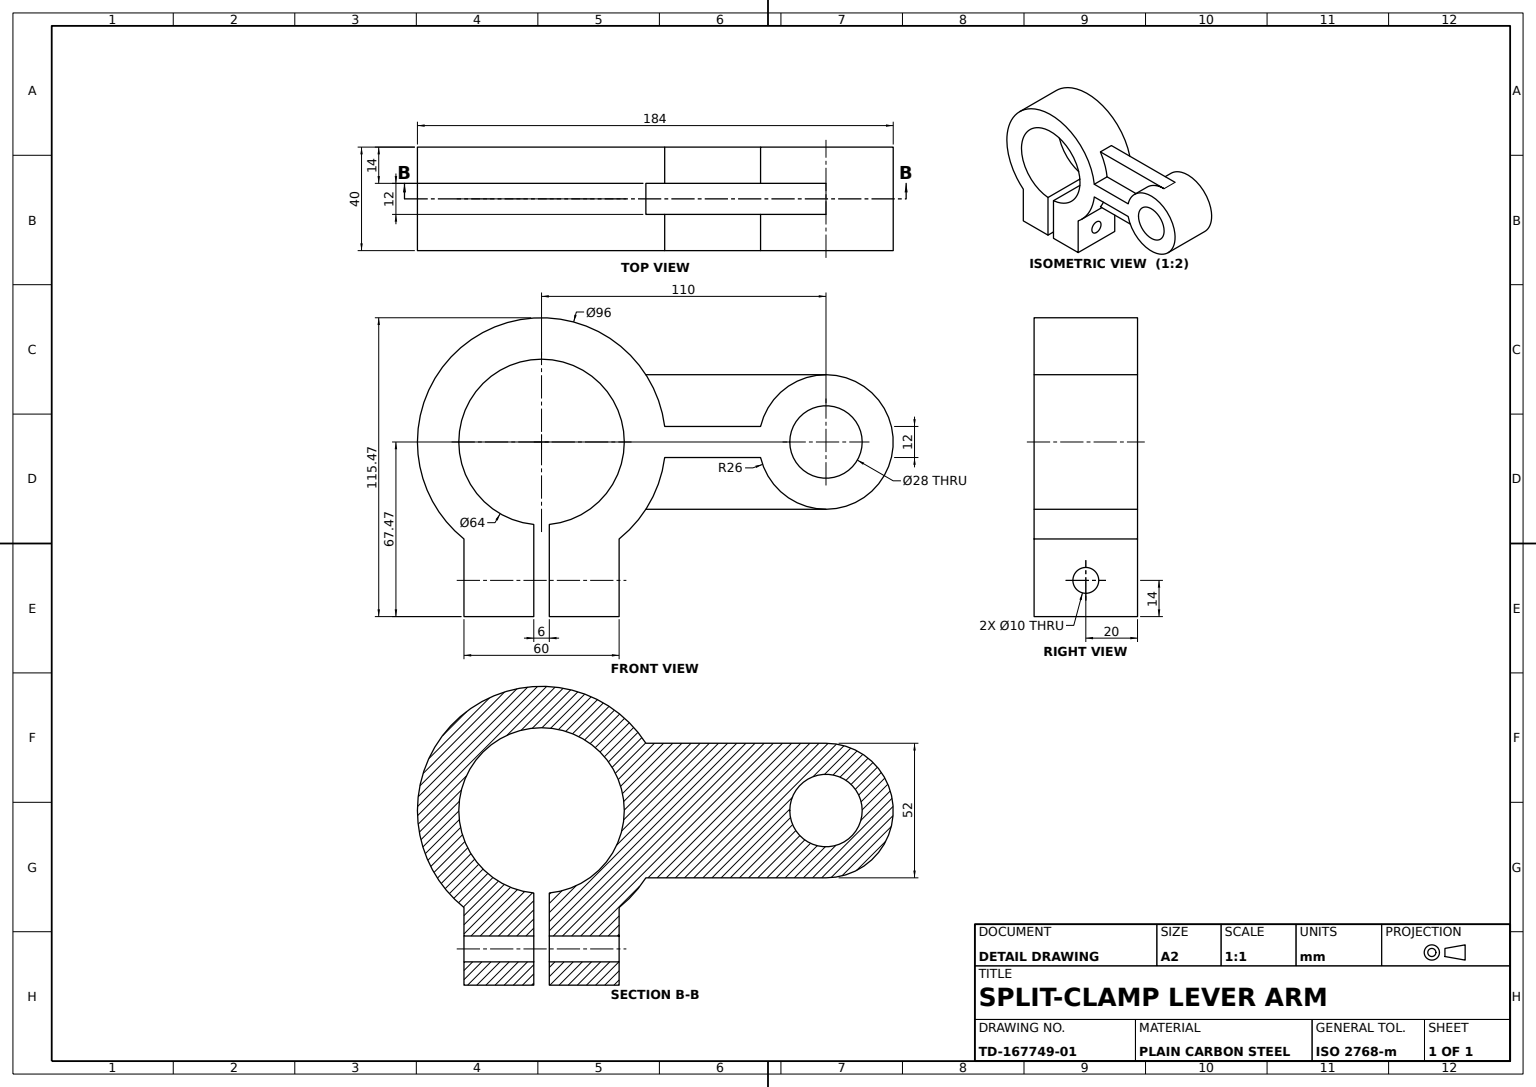
SolidWorks part; units mm, degrees
material "Plain Carbon Steel"
ref_plane "Front Plane" through (0, 0, 0) normal (0, 0, 1) x (1, 0, 0)
ref_plane "Top Plane" through (0, 0, 0) normal (0, 1, 0) x (1, 0, 0)
ref_plane "Right Plane" through (0, 0, 0) normal (1, 0, 0) x (0, 0, -1)
sketch "Clamp Ring Profile" plane through (0, 0, 0) normal (0, 0, 1) x (1, 0, 0)
  circle A0 centre (0, 0) radius 48
  dimension "D1" = 96
extrude "Clamp Ring Ø96" add sketch "Clamp Ring Profile" along normal mid plane 40
sketch "End Boss Profile" plane through (0, 0, 0) normal (0, 0, 1) x (1, 0, 0)
  circle A0 centre (110, 0) radius 26
  dimension "D1" = 52
  dimension "D2" = 110
extrude "End Boss Ø52" add sketch "End Boss Profile" along normal mid plane 40 separate body
sketch "Lever Web Profile" plane through (0, 0, 20) normal (0, 0, 1) x (1, 0, 0)
  line L1 (48, 6) -> (86.7905, 6)
  line L2 (86.7905, 6) -> (86.7905, -6)
  line L3 (86.7905, -6) -> (44, -6)
  line L4 (44, -6) -> (44, 6)
  line L5 (44, 6) -> (48, 6)
  circle A0 centre (0, 0) radius 48 construction
  dimension "D1" = 44
  dimension "D2" = 48
  dimension "D3" = 86.7905
  dimension "D4" = 6
  dimension "D5" = 6
extrude "Lever Web" add sketch "Lever Web Profile" against normal blind 40
sketch "Rib A Profile" plane through (0, 0, 0) normal (0, 0, 1) x (1, 0, 0)
  line L0 (110, 26) -> (40.3485, 26)
  line L1 (47.6235, 6) -> (84.7018, 6)
  arc A0 (84.7018, -6) -> (84.7018, 6) centre (110, 0) ccw construction
  arc A1 (47.6235, 6) -> (47.6235, -6) centre (0, 0) ccw construction
  arc A2 (40.3485, 26) -> (47.6235, 6) centre (0, 0) cw
  arc A3 (84.7018, 6) -> (110, 26) centre (110, 0) cw
extrude "Rib A" add sketch "Rib A Profile" along normal mid plane 12
sketch "Rib B Profile" plane through (0, 0, 0) normal (0, 0, 1) x (1, 0, 0)
  line L0 (110, -26) -> (40.276, -26)
  line L3 (84.7018, -6) -> (47.6235, -6)
  arc A0 (84.7018, -6) -> (84.7018, 6) centre (110, 0) ccw construction
  arc A1 (110, -26) -> (84.7018, -6) centre (110, 0) cw
  arc A2 (47.6235, -6) -> (40.276, -26) centre (-2.4571, 1.0487) cw
  dimension "D1" = 50.5743
  dimension "D2" = 69.724
extrude "Rib B" add sketch "Rib B Profile" along normal mid plane 12
sketch "Clamp Bore Profile" plane through (0, 0, 20) normal (0, 0, 1) x (1, 0, 0)
  circle A0 centre (0, 0) radius 32
  dimension "D1" = 64
extrude "Clamp Bore" cut sketch "Clamp Bore Profile" against normal blind 213
sketch "End Bore Profile" plane through (0, 0, 20) normal (0, 0, 1) x (1, 0, 0)
  circle A0 centre (110, 0) radius 14
  dimension "D1" = 28
extrude "End Bore" cut sketch "End Bore Profile" against normal blind 213
sketch "Clamp Lug Profile" plane through (0, 0, 20) normal (0, 0, 1) x (1, 0, 0)
  line L1 (0, -37.47) -> (30, -37.47)
  line L2 (30, -37.47) -> (30, -67.47)
  line L3 (30, -67.47) -> (-30, -67.47)
  line L4 (-30, -67.47) -> (-30, -37.47)
  line L5 (-30, -37.47) -> (0, -37.47)
  arc A3 (47.6235, 6) -> (47.6235, -6) centre (0, 0) ccw construction
  dimension "D1" = 17.6235
extrude "Clamp Lug" add sketch "Clamp Lug Profile" against normal blind 40
sketch "Clamp Slot Profile" plane through (0, 0, 20) normal (0, 0, 1) x (1, 0, 0)
  line L0 (0, -67.47) -> (3, -67.47)
  line L1 (-30, -67.47) -> (30, -67.47) construction
  line L2 (3, -67.47) -> (3, -25.3661)
  line L3 (3, -25.3661) -> (-3, -25.3661)
  line L4 (-3, -25.3661) -> (-3, -67.47)
  line L5 (-3, -67.47) -> (0, -67.47)
  line L6 (-30, -37.47) -> (-30, -67.47) construction
  dimension "D1" = 27
  dimension "D2" = 42.1039
extrude "Clamp Slot" cut sketch "Clamp Slot Profile" against normal blind 40
sketch "Clamp Screw Hole Profile" plane through (30, 0, 0) normal (1, 0, 0) x (0, 0, -1)
  line L0 (-20, -67.47) -> (-20, -37.47) construction
  line L1 (20, -67.47) -> (-20, -67.47) construction
  circle A0 centre (0, -53.47) radius 5
  dimension "D1" = 10
  dimension "D2" = 20
  dimension "D3" = 14
extrude "Clamp Screw Hole" cut sketch "Clamp Screw Hole Profile" against normal blind 105
